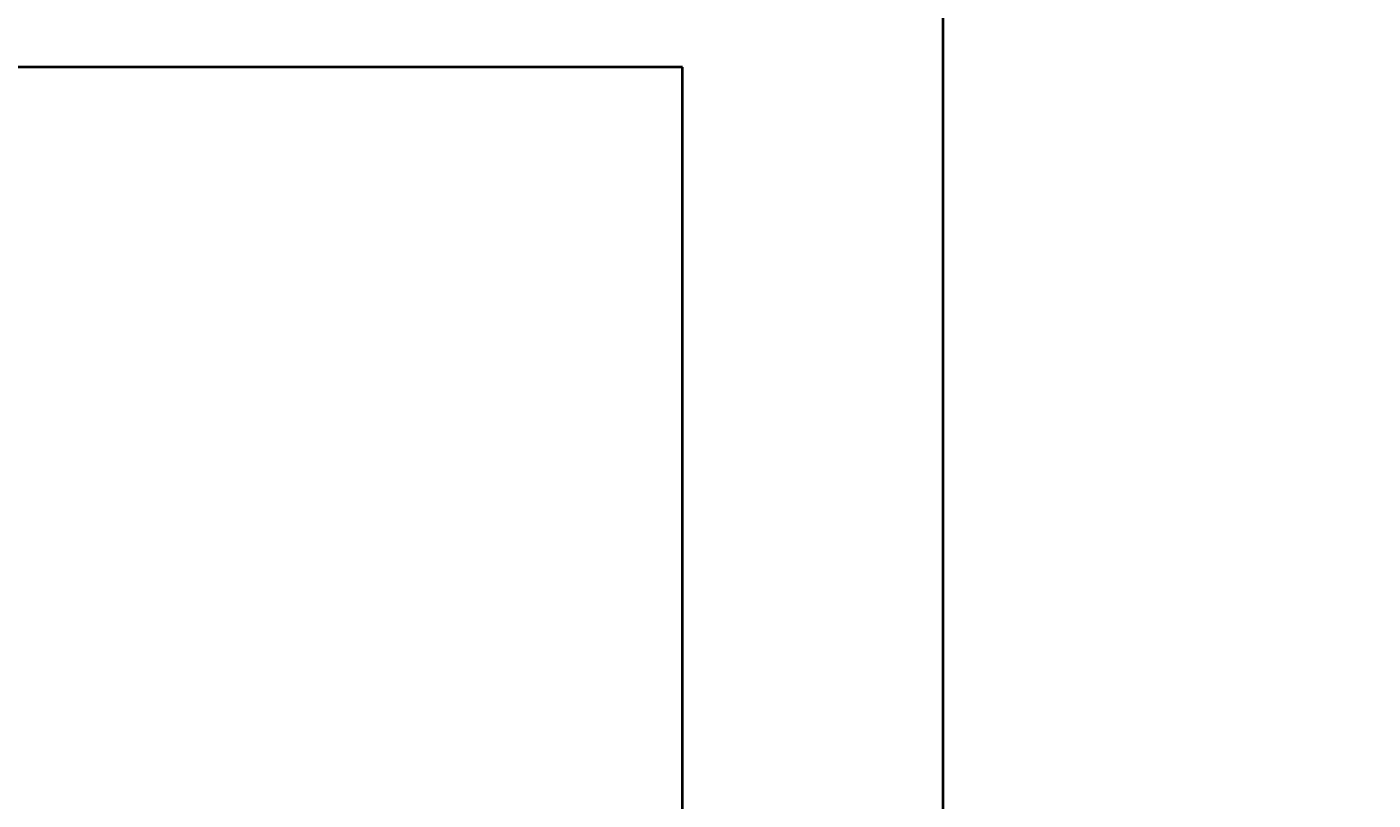
# Model space of a CAD drawing. Units: inches. Extents: x -301 to 715, y -607 to 364.
# Tile 123 of 141: x 101 to 148, y 276 to 303. Entities that reach past the tile are written whole.
import ezdxf

# ---------------------------------------------------------------- set-up
doc = ezdxf.new("R2010")
doc.units = ezdxf.units.IN
doc.header["$MEASUREMENT"] = 0
doc.layers.add('A-ANNO-DIMS', color=2, linetype='Continuous', lineweight=18)
doc.layers.add('A-WALL', color=3, linetype='Continuous', lineweight=40)
doc.styles.get("Standard").update_dxf_attribs({"font": 'arial.ttf'})
doc.dimstyles.get("Standard").update_dxf_attribs({"dimtxt": 0.18, "dimasz": 0.18, "dimexe": 0.18, "dimexo": 0.0625, "dimgap": 0.09, "dimtad": 0, "dimtih": 1, "dimtoh": 1, "dimdec": 1, "dimzin": 0, "dimdsep": 46, "dimlunit": 4, "dimtxsty": 'Standard', "dimcen": 0.09, "dimclrd": 3, "dimclre": 4, "dimclrt": 6, "dimadec": 0, "dimazin": 0, "dimtfac": 1, "dimtdec": 1, "dimtofl": 0, "dimtmove": 0, "dimatfit": 3, "dimfxl": 1, "dimtfill": 2, "dimtfillclr": 51, "dimtolj": 1, "dimtzin": 0, "dimarcsym": 0})

# ---------------------------------------------------------------- blocks, each defined once
blk = doc.blocks.new('*D153')
at = {"layer": 'A-ANNO-DIMS', "color": 4, "lineweight": -2, "transparency": 16777216}
for p, q in [((132.959, 310.182), (233.659, 310.182)), ((123.959, 193.182), (233.659, 193.182))]:
    blk.add_line(p, q, dxfattribs=at)
at = {"layer": 'A-ANNO-DIMS', "color": 3, "lineweight": -2, "transparency": 16777216}
for p, q in [((233.479, 310.002), (233.479, 251.864)), ((233.479, 193.362), (233.479, 251.5))]:
    blk.add_line(p, q, dxfattribs=at)
at = {"layer": 'A-ANNO-DIMS', "color": 3, "transparency": 16777216}
for points in [[(233.449, 310.002), (233.509, 310.002), (233.479, 310.182)], [(233.449, 193.362), (233.509, 193.362), (233.479, 193.182)]]:
    blk.add_solid(points, dxfattribs=at)
at = {"layer": 'Defpoints', "color": 0, "transparency": 16777216}
for p in [(132.897, 310.182), (123.897, 193.182), (233.479, 193.182)]:
    blk.add_point(p, dxfattribs=at)
at = {"layer": 'A-ANNO-DIMS', "color": 6, "transparency": 16777216, "insert": (233.479, 251.682), "char_height": 0.18, "attachment_point": 5, "bg_fill": 1, "box_fill_scale": 1.25, "bg_fill_color": 51, "bg_fill_transparency": 0}
blk.add_mtext('\\A1;9\'-9"', dxfattribs=at)

msp = doc.modelspace()

# ---------------------------------------------------------------- linework, layer by layer
at = {"layer": 'A-WALL'}
for p, q in [((132.897, 199.182), (132.897, 310.182)), ((123.897, 301.182), (15.897, 301.182)), ((123.897, 199.182), (123.897, 301.182))]:
    msp.add_line(p, q, dxfattribs=at)

# ---------------------------------------------------------------- dimensions: what is measured, and where the dimension line sits
at = {"layer": 'A-ANNO-DIMS'}
dim = msp.add_linear_dim(base=(233.479, 193.182), p1=(132.897, 310.182), p2=(123.897, 193.182), angle=90, dimstyle='Standard', override={"dimdec": 1, "dimlfac": 1, "dimrnd": 0, "dimzin": 1, "dimdsep": 46, "dimlunit": 4, "dimfrac": 2}, dxfattribs=at)
dim.commit()
dim.dimension.update_dxf_attribs({"geometry": '*D153', "text_midpoint": (233.479, 251.682)})

doc.saveas('drawing.dxf')
